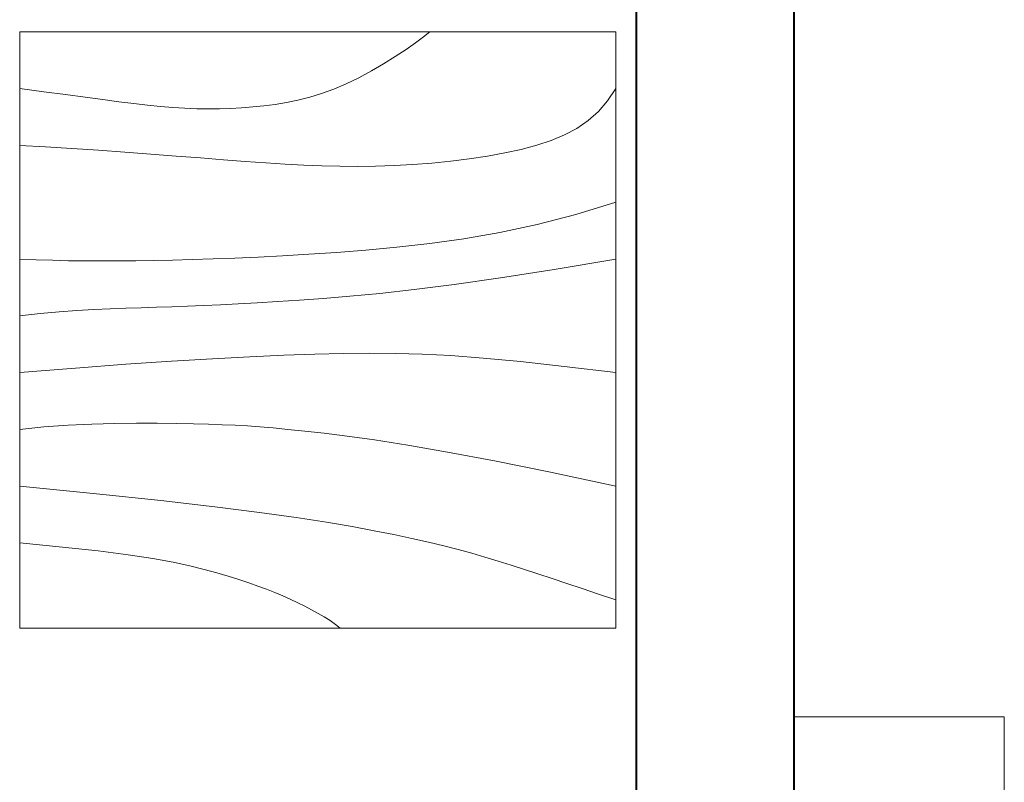
# Model space of a CAD drawing. Units: inches. Extents: x -301 to 715, y -607 to 364.
# Tile 115 of 141: x 89 to 145, y 149 to 192. Entities that reach past the tile are written whole.
import ezdxf

# ---------------------------------------------------------------- set-up
doc = ezdxf.new("R2010")
doc.units = ezdxf.units.IN
doc.header["$MEASUREMENT"] = 0
doc.linetypes.add('ACAD_ISO02W100', pattern=[15, 12, -3])
for name, color, linetype, lineweight in [('A-FURN', 8, 'Continuous', 18), ('A-GLAZ-OVHD', 2, 'ACAD_ISO02W100', 18), ('A-WALL', 3, 'Continuous', 40)]:
    doc.layers.add(name, color=color, linetype=linetype, lineweight=lineweight)

# ---------------------------------------------------------------- blocks, each defined once
blk = doc.blocks.new('Table - Square Woodgrain 42 x 42 in.')
blk.add_line((0, -42), (42, -42))
for points in [[(0, -4), (1.704, -4.2172), (3.2358, -4.4188), (4.615, -4.604), (5.8615, -4.7721), (6.9951, -4.9224), (8.0357, -5.0541), (9.0031, -5.1667), (9.9171, -5.2594), (10.7951, -5.3316), (11.6445, -5.3836), (12.4702, -5.4157), (13.277, -5.4283), (14.0698, -5.4217), (14.8535, -5.3964), (15.6331, -5.3526), (16.4133, -5.2908), (17.1986, -5.2103), (17.9913, -5.1062), (18.793, -4.9727), (19.6056, -4.8038), (20.4307, -4.5937), (21.2701, -4.3365), (22.1256, -4.0262), (22.9989, -3.6571), (23.888, -3.2272), (24.7756, -2.7516), (25.6408, -2.2491), (26.4624, -1.7387), (27.2195, -1.2395), (27.891, -0.7703), (28.456, -0.3501), (28.8934, 0.002)], [(0, -42), (0, 0), (42, 0), (42, -42)], [(0, -8), (1.8203, -8.1001), (3.6741, -8.2149), (5.5411, -8.3408), (7.4011, -8.4741), (9.2339, -8.6112), (11.0193, -8.7484), (12.7371, -8.8821), (14.3671, -9.0086), (15.8954, -9.1246), (17.3337, -9.2278), (18.6997, -9.3159), (20.0116, -9.387), (21.2871, -9.4389), (22.5442, -9.4696), (23.8008, -9.477), (25.0749, -9.459), (26.3791, -9.4137), (27.7049, -9.3403), (29.0383, -9.2382), (30.3655, -9.1068), (31.6728, -8.9455), (32.9461, -8.7535), (34.1717, -8.5304), (35.3358, -8.2756), (36.4268, -7.9863), (37.443, -7.6521), (38.3849, -7.2603), (39.253, -6.7986), (40.048, -6.2542), (40.7705, -5.6147), (41.421, -4.8674), (42, -4)], [(42, -12), (39.1784, -12.8621), (36.4519, -13.5654), (33.8246, -14.1294), (31.3004, -14.5731), (28.8832, -14.9161), (26.577, -15.1775), (24.3858, -15.3768), (22.3136, -15.5332), (20.3622, -15.6632), (18.5254, -15.7718), (16.7947, -15.8612), (15.1618, -15.9338), (13.6183, -15.9916), (12.1558, -16.0369), (10.7659, -16.0718), (9.4403, -16.0987), (8.1703, -16.1191), (6.9461, -16.1325), (5.7577, -16.1377), (4.595, -16.1335), (3.4479, -16.1188), (2.3064, -16.0924), (1.1604, -16.0532), (0, -16)], [(42, -16), (37.6529, -16.7365), (33.8802, -17.329), (30.6179, -17.7961), (27.8015, -18.1561), (25.3668, -18.4275), (23.2497, -18.6288), (21.3859, -18.7785), (19.7111, -18.8949), (18.1693, -18.9939), (16.7375, -19.0795), (15.401, -19.1534), (14.1449, -19.217), (12.9544, -19.2717), (11.8148, -19.3191), (10.7113, -19.3606), (9.6291, -19.3976), (8.5534, -19.4323), (7.47, -19.4689), (6.3643, -19.5122), (5.222, -19.5672), (4.0288, -19.6386), (2.7703, -19.7313), (1.4321, -19.8501), (0, -20)], [(0, -24), (3.9243, -23.6805), (7.4766, -23.4138), (10.6891, -23.1954), (13.5943, -23.0205), (16.2247, -22.8847), (18.6125, -22.7832), (20.7903, -22.7116), (22.7903, -22.6651), (24.6563, -22.642), (26.4764, -22.6507), (28.35, -22.7024), (30.3766, -22.8084), (32.6555, -22.98), (35.2861, -23.2283), (38.3678, -23.5645), (42, -24)], [(42, -32), (37.392, -31.017), (33.4585, -30.2231), (30.1291, -29.5949), (27.3334, -29.109), (25.0009, -28.742), (23.0612, -28.4707), (21.4439, -28.2716), (20.0786, -28.1215), (18.8998, -28.0002), (17.8609, -27.9014), (16.9206, -27.8219), (16.0371, -27.7588), (15.1691, -27.709), (14.2748, -27.6693), (13.3128, -27.6368), (12.2415, -27.6083), (11.0295, -27.5824), (9.6867, -27.5643), (8.233, -27.5608), (6.6884, -27.5787), (5.0728, -27.6248), (3.4062, -27.7058), (1.7086, -27.8286), (0, -28)], [(0, -32), (5.4026, -32.5358), (9.9494, -33.019), (13.7424, -33.4553), (16.8834, -33.8505), (19.4743, -34.2106), (21.6171, -34.5413), (23.4136, -34.8486), (24.9657, -35.1382), (26.3614, -35.4156), (27.6332, -35.6841), (28.7995, -35.9467), (29.8788, -36.2064), (30.8897, -36.4661), (31.8507, -36.7288), (32.7802, -36.9973), (33.6968, -37.2747), (34.6175, -37.5635), (35.5531, -37.8651), (36.5128, -38.1805), (37.506, -38.5108), (38.5421, -38.8568), (39.6302, -39.2197), (40.7797, -39.6004), (42, -40)], [(0, -36), (3.0098, -36.2857), (5.5354, -36.5643), (7.6368, -36.8359), (9.374, -37.1009), (10.807, -37.3597), (11.9957, -37.6126), (13.0002, -37.8599), (13.8804, -38.102), (14.6874, -38.3393), (15.4365, -38.5729), (16.1338, -38.8041), (16.7858, -39.0341), (17.3987, -39.264), (17.9787, -39.4952), (18.5322, -39.7288), (19.0655, -39.9662), (19.5832, -40.2081), (20.0842, -40.4544), (20.5657, -40.7046), (21.0249, -40.9581), (21.459, -41.2144), (21.8653, -41.4731), (22.2409, -41.7335), (22.5831, -41.9951)]]:
    blk.add_lwpolyline(points)
blk = doc.blocks.new('WIN-SHADE-50')
at = {"ltscale": 1.5}
for p, q in [((0, 0), (0, 12)), ((50, 12), (0, 12)), ((5, 0), (0, 0))]:
    blk.add_line(p, q, dxfattribs=at)

msp = doc.modelspace()

# ---------------------------------------------------------------- linework, layer by layer
at = {"layer": 'A-WALL'}
for p, q in [((132.897, -9.818), (132.897, 199.182)), ((123.897, -9.818), (123.897, 193.182))]:
    msp.add_line(p, q, dxfattribs=at)

# ---------------------------------------------------------------- block references
at = {"layer": 'A-FURN', "xscale": 0.8107193059798699, "yscale": 0.8107193059798699, "zscale": 0.8107193059798699}
msp.add_blockref('Table - Square Woodgrain 42 x 42 in.', (88.66, 191.795), dxfattribs=at)
at = {"layer": 'A-GLAZ-OVHD', "rotation": 270.0000000000001}
msp.add_blockref('WIN-SHADE-50', (132.896, 152.682), dxfattribs=at)

doc.saveas('drawing.dxf')
